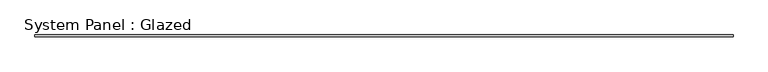
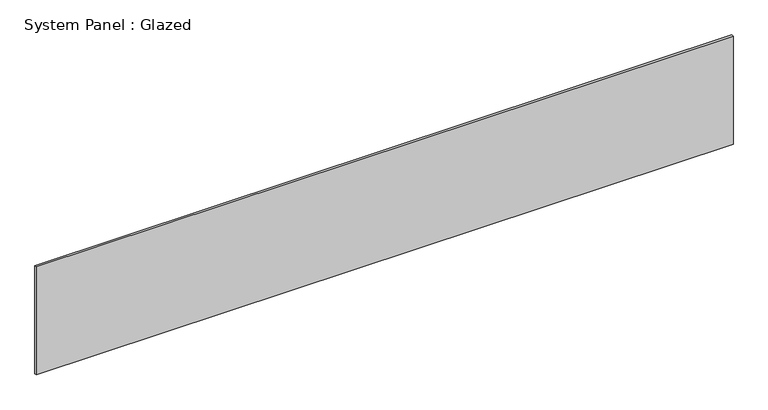
"""IFC4 building model written with IfcOpenShell, lengths in millimetres: plate geometry, System Panel : Glazed."""

from ifc_helpers import new_model, si_unit, origin, origin_with_axes, place, context, project, spatial, polyline, outline, extrude, source, transform, mapped, element, save


def system_panel_glazed_75d2b8fb(model_context):
    return source(origin(), model_context, "Body", "SweptSolid", [
        extrude(outline(polyline([(4648.2, 19.05), (-4648.2, 19.05), (-4648.2, 44.45), (4648.2, 44.45), (4648.2, 19.05)])), origin_with_axes(), (0.0, 0.0, 1.0), 1524.0),
    ])


if __name__ == "__main__":
    model = new_model("IFC4")
    model_context = context("Model", 3, world=origin())
    ifc_project = project(units=[si_unit("LENGTHUNIT", "METRE", prefix="MILLI")], contexts=[model_context])
    site = spatial("IfcSite", under=ifc_project)
    building = spatial("IfcBuilding", under=site)
    placement = place(None, origin())
    system_panel_glazed_shape = system_panel_glazed_75d2b8fb(model_context)
    element("IfcPlate", 1, ObjectType="System Panel : Glazed", at=placement, inside=building, context=model_context, shape_type="MappedRepresentation", body=[
        mapped(system_panel_glazed_shape, transform((0.0, 0.0, 0.0), x_axis=(1.0, 0.0, 0.0), y_axis=(0.0, 1.0, 0.0), z_axis=(0.0, 0.0, 1.0))),
    ])
    save(model, "model.ifc")

# Revit data of these elements
# Type "System Panel : Glazed"
#   Construction Type Id = "GSP4R"
#   Analytic Construction = "1/8 in Pilkington single glazing"
#   Visual Light Transmittance = 0.9
#   Solar Heat Gain Coefficient = 0.86
#   Heat Transfer Coefficient (U) = 1.18115 BTU/(h·ft²·°F)
# Element 1 (IfcPlate, "System Panel : Glazed")
#   Materials on its faces: "Glass"
# Materials
#   "Glass": class "Glass", colour RGB 0 128 192, transparency 0.75, Description = "Soda Lime Glass", Cost = 0
